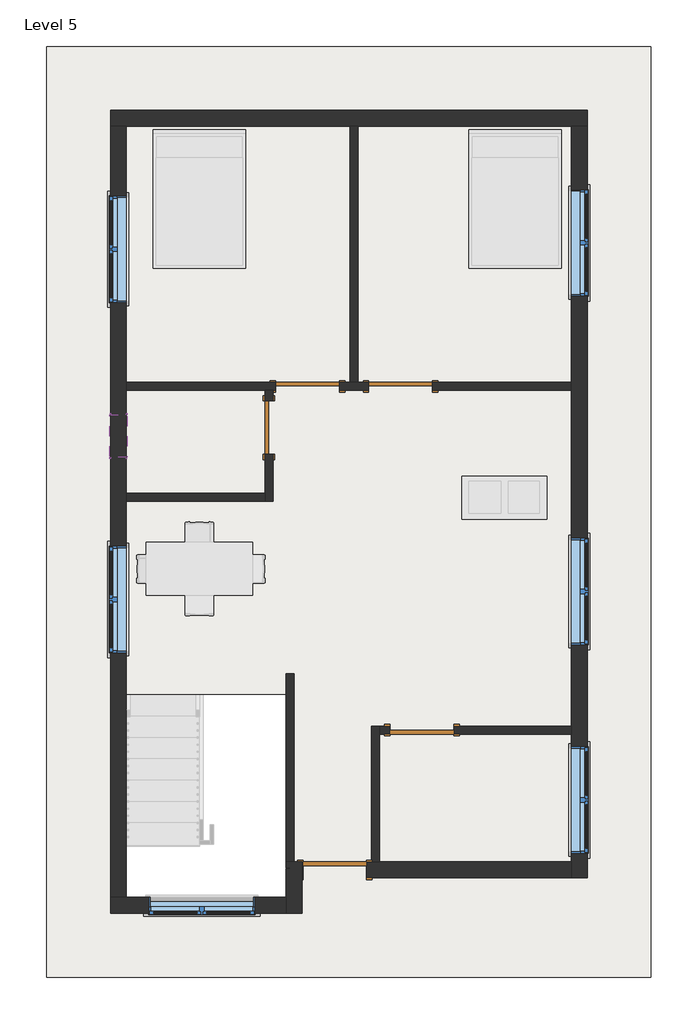
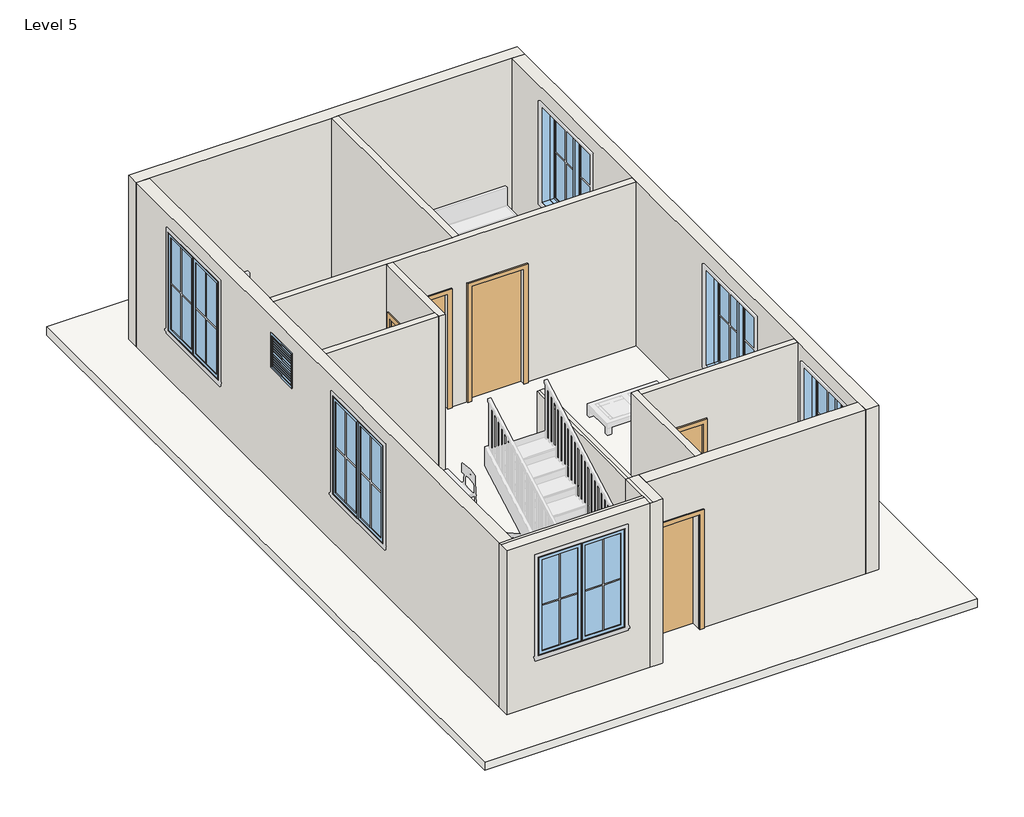
# One storey, part 1 of 3: 13 walls, 7 windows, 5 doors, 1 roof.
"""IFC4 building model written with IfcOpenShell, lengths in millimetres."""

from ifc_helpers import new_model, si_unit, frame, origin, place, context, project, spatial, polyline, outline, extrude, faceted_brep, transform, mapped, element, save
from components import door_214872d5, single_flush_door_3_e5f9f3c4, single_flush_door_3_305aa2a5, single_flush_door_3_0ca8825f, window_casement_double_win_5_f93960c7, window_f2d8fef0

model = new_model("IFC4")

# Units and contexts
model_context = context("Model", 3, world=origin())
ifc_project = project(units=[si_unit("LENGTHUNIT", "METRE", prefix="MILLI")], contexts=[model_context])

# Site, building, storey
site = spatial("IfcSite", under=ifc_project)
building = spatial("IfcBuilding", under=site)
storey = spatial("IfcBuildingStorey", under=building, Name="Level 5", Elevation=12649.2)

# Doors
placement = place(None, origin())
door_shape = door_214872d5(model_context)
element("IfcDoor", 1, ObjectType="Single-Flush : DOOR 2'6\"", at=placement, inside=storey, context=model_context, shape_type="MappedRepresentation", body=[
    mapped(door_shape, transform((-2193.930864, 251.0919982, 12649.2), x_axis=(0.0, 1.0, 0.0), y_axis=(-1.0, 0.0, 0.0), z_axis=(0.0, 0.0, 1.0))),
])
single_flush_door_3_shape = single_flush_door_3_e5f9f3c4(model_context)
element("IfcDoor", 2, ObjectType="Single-Flush : DOOR 3'", at=placement, inside=storey, context=model_context, shape_type="MappedRepresentation", body=[
    mapped(single_flush_door_3_shape, transform((-1641.3962678, 841.6419982, 12649.2), x_axis=(1.0, 0.0, 0.0), y_axis=(0.0, 1.0, 0.0), z_axis=(0.0, 0.0, 1.0))),
])
element("IfcDoor", 3, ObjectType="Single-Flush : DOOR 3'", at=placement, inside=storey, context=model_context, shape_type="MappedRepresentation", body=[
    mapped(single_flush_door_3_shape, transform((-3.180864, -4073.2580018, 12649.2), x_axis=(-1.0, 0.0, 0.0), y_axis=(0.0, -1.0, 0.0), z_axis=(0.0, 0.0, 1.0))),
])
single_flush_door_3_2_shape = single_flush_door_3_305aa2a5(model_context)
element("IfcDoor", 4, ObjectType="Single-Flush : DOOR 3'", at=placement, inside=storey, context=model_context, shape_type="MappedRepresentation", body=[
    mapped(single_flush_door_3_2_shape, transform((-307.980864, 841.6419982, 12649.2), x_axis=(-1.0, 0.0, 0.0), y_axis=(0.0, -1.0, 0.0), z_axis=(0.0, 0.0, 1.0))),
])
single_flush_door_3_3_shape = single_flush_door_3_0ca8825f(model_context)
element("IfcDoor", 5, ObjectType="Single-Flush : DOOR 3'", at=placement, inside=storey, context=model_context, shape_type="MappedRepresentation", body=[
    mapped(single_flush_door_3_3_shape, transform((-1250.955864, -6073.5080018, 12649.2), x_axis=(1.0, 0.0, 0.0), y_axis=(0.0, 1.0, 0.0), z_axis=(0.0, 0.0, 1.0))),
])

# Roof
element("IfcRoof", 6, ObjectType="ROOF 6\"", at=placement, inside=storey, context=model_context, shape_type="SweptSolid", body=[
    extrude(outline(polyline([(3273.419136, 5699.3919982), (3273.419136, -7610.2080018), (-5375.280864, -7610.2080018), (-5375.280864, 5699.3919982), (3273.419136, 5699.3919982)]), holes=[polyline([(-1895.480864, -3571.6080018), (-4232.280864, -3571.6080018), (-4232.280864, -6518.0080018), (-1895.480864, -6518.0080018), (-1895.480864, -3571.6080018)])]), frame((0.0, 0.0, 12496.8), z_axis=(0.0, 0.0, 1.0), x_axis=(1.0, 0.0, 0.0)), (0.0, 0.0, 1.0), 152.4),
])

# Walls
element("IfcWall", 7, ObjectType="WALL 4.5\"", at=placement, inside=storey, context=model_context, shape_type="SweptSolid", body=[
    extrude(outline(polyline([(-1031.880864, 898.7919982), (-1031.880864, 4556.3919982), (-917.580864, 4556.3919982), (-917.580864, 898.7919982), (-1031.880864, 898.7919982)])), frame((0.0, 0.0, 12649.2), z_axis=(0.0, 0.0, 1.0), x_axis=(1.0, 0.0, 0.0)), (0.0, 0.0, 1.0), 3048.0),
])
element("IfcWall", 8, ObjectType="WALL 4.5\"", at=placement, inside=storey, context=model_context, shape_type="Brep", body=[
    faceted_brep([(-765.180864, 898.7919982, 14782.8), (-765.180864, 898.7919982, 12649.2), (-917.580864, 898.7919982, 12649.2), (-1031.880864, 898.7919982, 12649.2), (-1184.1962678, 898.7919982, 12649.2), (-1184.1962678, 898.7919982, 14782.8), (-2098.5962678, 898.7919982, 14782.8), (-2098.5962678, 898.7919982, 12649.2), (-4232.280864, 898.7919982, 12649.2), (-4232.280864, 898.7919982, 15697.2), (-1031.880864, 898.7919982, 15697.2), (-917.580864, 898.7919982, 15697.2), (2130.419136, 898.7919982, 15697.2), (2130.419136, 898.7919982, 12649.2), (149.219136, 898.7919982, 12649.2), (149.219136, 898.7919982, 14782.8), (-1184.1962678, 784.4919982, 12649.2), (-765.180864, 784.4919982, 12649.2), (-765.180864, 784.4919982, 14782.8), (149.219136, 784.4919982, 14782.8), (149.219136, 784.4919982, 12649.2), (2130.419136, 784.4919982, 12649.2), (2130.419136, 784.4919982, 15697.2), (-2136.780864, 784.4919982, 15697.2), (-2251.080864, 784.4919982, 15697.2), (-4232.280864, 784.4919982, 15697.2), (-4232.280864, 784.4919982, 12649.2), (-2251.080864, 784.4919982, 12649.2), (-2136.780864, 784.4919982, 12649.2), (-2098.5962678, 784.4919982, 12649.2), (-2098.5962678, 784.4919982, 14782.8), (-1184.1962678, 784.4919982, 14782.8)], [[[0, 1, 2, 3, 4, 5, 6, 7, 8, 9, 10, 11, 12, 13, 14, 15]], [[16, 17, 18, 19, 20, 21, 22, 23, 24, 25, 26, 27, 28, 29, 30, 31]], [[29, 28, 27, 26, 8, 7]], [[14, 13, 21, 20]], [[4, 3, 2, 1, 17, 16]], [[13, 12, 22, 21]], [[9, 8, 26, 25]], [[5, 4, 16, 31]], [[6, 5, 31, 30]], [[7, 6, 30, 29]], [[18, 17, 1, 0]], [[19, 18, 0, 15]], [[20, 19, 15, 14]], [[12, 11, 10, 9, 25, 24, 23, 22]]]),
])
element("IfcWall", 9, ObjectType="WALL 4.5\"", at=placement, inside=storey, context=model_context, shape_type="Brep", body=[
    faceted_brep([(-2251.080864, 784.4919982, 12649.2), (-2251.080864, 632.0919982, 12649.2), (-2251.080864, 632.0919982, 14782.8), (-2251.080864, -129.9080018, 14782.8), (-2251.080864, -129.9080018, 12649.2), (-2251.080864, -688.7080018, 12649.2), (-2251.080864, -803.0080018, 12649.2), (-2251.080864, -803.0080018, 15697.2), (-2251.080864, -688.7080018, 15697.2), (-2251.080864, 784.4919982, 15697.2), (-2136.780864, 632.0919982, 14782.8), (-2136.780864, 632.0919982, 12649.2), (-2136.780864, 784.4919982, 12649.2), (-2136.780864, 784.4919982, 15697.2), (-2136.780864, -803.0080018, 15697.2), (-2136.780864, -803.0080018, 12649.2), (-2136.780864, -129.9080018, 12649.2), (-2136.780864, -129.9080018, 14782.8)], [[[0, 1, 2, 3, 4, 5, 6, 7, 8, 9]], [[10, 11, 12, 13, 14, 15, 16, 17]], [[16, 15, 6, 5, 4]], [[12, 11, 1, 0]], [[0, 9, 13, 12]], [[7, 6, 15, 14]], [[2, 1, 11, 10]], [[3, 2, 10, 17]], [[4, 3, 17, 16]], [[9, 8, 7, 14, 13]]]),
])
element("IfcWall", 10, ObjectType="WALL 4.5\"", at=placement, inside=storey, context=model_context, shape_type="SweptSolid", body=[
    extrude(outline(polyline([(-4232.280864, -688.7080018), (-2251.080864, -688.7080018), (-2251.080864, -803.0080018), (-4232.280864, -803.0080018), (-4232.280864, -688.7080018)])), frame((0.0, 0.0, 12649.2), z_axis=(0.0, 0.0, 1.0), x_axis=(1.0, 0.0, 0.0)), (0.0, 0.0, 1.0), 3048.0),
])
element("IfcWall", 11, ObjectType="WALL 4.5\"", at=placement, inside=storey, context=model_context, shape_type="Brep", body=[
    faceted_brep([(-1831.980864, -5959.2080018, 12649.2), (-1831.980864, -3266.8080018, 12649.2), (-1831.980864, -3266.8080018, 15697.2), (-1831.980864, -5959.2080018, 15697.2), (-1946.280864, -5959.2080018, 12649.2), (-1946.280864, -5959.2080018, 15697.2), (-1946.280864, -3266.8080018, 15697.2), (-1946.280864, -3266.8080018, 12649.2), (-1895.480864, -3266.8080018, 15697.2), (-1895.480864, -5959.2080018, 15697.2), (-1895.480864, -3571.6080018, 15697.2)], [[[0, 1, 2, 3]], [[4, 5, 6, 7]], [[1, 0, 4, 7]], [[2, 1, 7, 6, 8]], [[0, 3, 9, 5, 4]], [[3, 2, 8, 10, 9]], [[8, 6, 5, 9, 10]]]),
])
element("IfcWall", 12, ObjectType="WALL 4.5\"", at=placement, inside=storey, context=model_context, shape_type="Brep", body=[
    faceted_brep([(-612.780864, -5959.2080018, 12649.2), (-612.780864, -4130.4080018, 12649.2), (-612.780864, -4016.1080018, 12649.2), (-612.780864, -4016.1080018, 15697.2), (-612.780864, -4130.4080018, 15697.2), (-612.780864, -5959.2080018, 15697.2), (-727.080864, -5959.2080018, 12649.2), (-727.080864, -5959.2080018, 15697.2), (-727.080864, -4016.1080018, 15697.2), (-727.080864, -4016.1080018, 12649.2)], [[[0, 1, 2, 3, 4, 5]], [[6, 7, 8, 9]], [[2, 1, 0, 6, 9]], [[0, 5, 7, 6]], [[3, 2, 9, 8]], [[5, 4, 3, 8, 7]]]),
])
element("IfcWall", 13, ObjectType="WALL 4.5\"", at=placement, inside=storey, context=model_context, shape_type="SweptSolid", body=[
    extrude(outline(polyline([(12649.2, -612.780864), (12649.2, -460.380864), (14782.8, -460.380864), (14782.8, 454.019136), (12649.2, 454.019136), (12649.2, 2130.419136), (15697.2, 2130.419136), (15697.2, -612.780864), (12649.2, -612.780864)])), frame((0.0, -4130.4080018, 0.0), z_axis=(0.0, 1.0, 0.0), x_axis=(0.0, 0.0, 1.0)), (0.0, 0.0, 1.0), 114.3),
])
element("IfcWall", 14, ObjectType="WALL 9\"", at=placement, inside=storey, context=model_context, shape_type="Brep", body=[
    faceted_brep([(-4460.880864, 4556.3919982, 12649.2), (-4232.280864, 4556.3919982, 12649.2), (-1031.880864, 4556.3919982, 12649.2), (-917.580864, 4556.3919982, 12649.2), (2130.419136, 4556.3919982, 12649.2), (2359.019136, 4556.3919982, 12649.2), (2359.019136, 4556.3919982, 15697.2), (2130.419136, 4556.3919982, 15697.2), (-917.580864, 4556.3919982, 15697.2), (-1031.880864, 4556.3919982, 15697.2), (-4232.280864, 4556.3919982, 15697.2), (-4460.880864, 4556.3919982, 15697.2), (-4460.880864, 4784.9919982, 12649.2), (-4460.880864, 4784.9919982, 15697.2), (2359.019136, 4784.9919982, 15697.2), (2359.019136, 4784.9919982, 12649.2)], [[[0, 1, 2, 3, 4, 5, 6, 7, 8, 9, 10, 11]], [[12, 13, 14, 15]], [[5, 4, 3, 2, 1, 0, 12, 15]], [[6, 5, 15, 14]], [[0, 11, 13, 12]], [[11, 10, 9, 8, 7, 6, 14, 13]]]),
])
element("IfcWall", 15, ObjectType="WALL 9\"", at=placement, inside=storey, context=model_context, shape_type="Brep", body=[
    faceted_brep([(2130.419136, 4556.3919982, 12649.2), (2130.419136, 898.7919982, 12649.2), (2130.419136, 784.4919982, 12649.2), (2130.419136, -4016.1080018, 12649.2), (2130.419136, -4130.4080018, 12649.2), (2130.419136, -5959.2080018, 12649.2), (2130.419136, -6187.8080018, 12649.2), (2130.419136, -6187.8080018, 15697.2), (2130.419136, -5959.2080018, 15697.2), (2130.419136, -4130.4080018, 15697.2), (2130.419136, -4016.1080018, 15697.2), (2130.419136, 784.4919982, 15697.2), (2130.419136, 898.7919982, 15697.2), (2130.419136, 4556.3919982, 15697.2), (2130.419136, -5835.3830018, 15392.4), (2130.419136, -5835.3830018, 13563.6), (2130.419136, -4311.3830018, 13563.6), (2130.419136, -4311.3830018, 15392.4), (2130.419136, -2854.0580018, 15392.4), (2130.419136, -2854.0580018, 13563.6), (2130.419136, -1330.0580018, 13563.6), (2130.419136, -1330.0580018, 15392.4), (2130.419136, 2130.6919982, 15392.4), (2130.419136, 2130.6919982, 13563.6), (2130.419136, 3654.6919982, 13563.6), (2130.419136, 3654.6919982, 15392.4), (2359.019136, 4556.3919982, 12649.2), (2359.019136, 4556.3919982, 15697.2), (2359.019136, -6187.8080018, 15697.2), (2359.019136, -6187.8080018, 12649.2), (2359.019136, -5835.3830018, 15392.4), (2359.019136, -4311.3830018, 15392.4), (2359.019136, -4311.3830018, 13563.6), (2359.019136, -5835.3830018, 13563.6), (2359.019136, -2854.0580018, 15392.4), (2359.019136, -1330.0580018, 15392.4), (2359.019136, -1330.0580018, 13563.6), (2359.019136, -2854.0580018, 13563.6), (2359.019136, 2130.6919982, 15392.4), (2359.019136, 3654.6919982, 15392.4), (2359.019136, 3654.6919982, 13563.6), (2359.019136, 2130.6919982, 13563.6)], [[[0, 1, 2, 3, 4, 5, 6, 7, 8, 9, 10, 11, 12, 13], [14, 15, 16, 17], [18, 19, 20, 21], [22, 23, 24, 25]], [[26, 27, 28, 29], [30, 31, 32, 33], [34, 35, 36, 37], [38, 39, 40, 41]], [[6, 5, 4, 3, 2, 1, 0, 26, 29]], [[0, 13, 27, 26]], [[7, 6, 29, 28]], [[15, 14, 30, 33]], [[16, 15, 33, 32]], [[17, 16, 32, 31]], [[14, 17, 31, 30]], [[19, 18, 34, 37]], [[20, 19, 37, 36]], [[21, 20, 36, 35]], [[18, 21, 35, 34]], [[23, 22, 38, 41]], [[24, 23, 41, 40]], [[25, 24, 40, 39]], [[22, 25, 39, 38]], [[13, 12, 11, 10, 9, 8, 7, 28, 27]]]),
])
element("IfcWall", 16, ObjectType="WALL 9\"", at=placement, inside=storey, context=model_context, shape_type="Brep", body=[
    faceted_brep([(2130.419136, -5959.2080018, 12649.2), (-612.780864, -5959.2080018, 12649.2), (-727.080864, -5959.2080018, 12649.2), (-793.755864, -5959.2080018, 12649.2), (-793.755864, -5959.2080018, 14782.8), (-1708.155864, -5959.2080018, 14782.8), (-1708.155864, -5959.2080018, 12649.2), (-1717.680864, -5959.2080018, 12649.2), (-1717.680864, -5959.2080018, 15697.2), (-727.080864, -5959.2080018, 15697.2), (-612.780864, -5959.2080018, 15697.2), (2130.419136, -5959.2080018, 15697.2), (-793.755864, -6187.8080018, 14782.8), (-793.755864, -6187.8080018, 12649.2), (2130.419136, -6187.8080018, 12649.2), (2130.419136, -6187.8080018, 15697.2), (-1717.680864, -6187.8080018, 15697.2), (-1717.680864, -6187.8080018, 12649.2), (-1708.155864, -6187.8080018, 12649.2), (-1708.155864, -6187.8080018, 14782.8)], [[[0, 1, 2, 3, 4, 5, 6, 7, 8, 9, 10, 11]], [[12, 13, 14, 15, 16, 17, 18, 19]], [[18, 17, 7, 6]], [[14, 13, 3, 2, 1, 0]], [[0, 11, 15, 14]], [[8, 7, 17, 16]], [[4, 3, 13, 12]], [[5, 4, 12, 19]], [[6, 5, 19, 18]], [[11, 10, 9, 8, 16, 15]]]),
])
element("IfcWall", 17, ObjectType="WALL 9\"", at=placement, inside=storey, context=model_context, shape_type="Brep", body=[
    faceted_brep([(-1946.280864, -5959.2080018, 12649.2), (-1946.280864, -6467.2080018, 12649.2), (-1946.280864, -6695.8080018, 12649.2), (-1946.280864, -6695.8080018, 15697.2), (-1946.280864, -6467.2080018, 15697.2), (-1946.280864, -5959.2080018, 15697.2), (-1717.680864, -5959.2080018, 12649.2), (-1717.680864, -5959.2080018, 15697.2), (-1717.680864, -6187.8080018, 15697.2), (-1717.680864, -6695.8080018, 15697.2), (-1717.680864, -6695.8080018, 12649.2), (-1717.680864, -6187.8080018, 12649.2), (-1831.980864, -5959.2080018, 12649.2), (-1895.480864, -5959.2080018, 15697.2), (-1831.980864, -5959.2080018, 15697.2), (-1895.480864, -6695.8080018, 15697.2), (-1895.480864, -6518.0080018, 15697.2)], [[[0, 1, 2, 3, 4, 5]], [[6, 7, 8, 9, 10, 11]], [[2, 1, 0, 12, 6, 11, 10]], [[0, 5, 13, 14, 7, 6, 12]], [[3, 2, 10, 9, 15]], [[5, 4, 3, 15, 16, 13]], [[15, 9, 8, 7, 14, 13, 16]]]),
])
element("IfcWall", 18, ObjectType="WALL 9\"", at=placement, inside=storey, context=model_context, shape_type="Brep", body=[
    faceted_brep([(-1946.280864, -6467.2080018, 12649.2), (-4232.280864, -6467.2080018, 12649.2), (-4460.880864, -6467.2080018, 12649.2), (-4460.880864, -6467.2080018, 15697.2), (-4232.280864, -6467.2080018, 15697.2), (-1946.280864, -6467.2080018, 15697.2), (-3914.780864, -6467.2080018, 15392.4), (-3914.780864, -6467.2080018, 13563.6), (-2390.780864, -6467.2080018, 13563.6), (-2390.780864, -6467.2080018, 15392.4), (-1946.280864, -6695.8080018, 12649.2), (-1946.280864, -6695.8080018, 15697.2), (-4460.880864, -6695.8080018, 15697.2), (-4460.880864, -6695.8080018, 12649.2), (-3914.780864, -6695.8080018, 15392.4), (-2390.780864, -6695.8080018, 15392.4), (-2390.780864, -6695.8080018, 13563.6), (-3914.780864, -6695.8080018, 13563.6), (-1946.280864, -6518.0080018, 15697.2), (-4460.880864, -6518.0080018, 15697.2), (-4232.280864, -6518.0080018, 15697.2)], [[[0, 1, 2, 3, 4, 5], [6, 7, 8, 9]], [[10, 11, 12, 13], [14, 15, 16, 17]], [[2, 1, 0, 10, 13]], [[0, 5, 18, 11, 10]], [[3, 2, 13, 12, 19]], [[7, 6, 14, 17]], [[8, 7, 17, 16]], [[9, 8, 16, 15]], [[6, 9, 15, 14]], [[5, 4, 3, 19, 20, 18]], [[19, 12, 11, 18, 20]]]),
])
element("IfcWall", 19, ObjectType="WALL 9\"", at=placement, inside=storey, context=model_context, shape_type="Brep", body=[
    faceted_brep([(-4232.280864, -6467.2080018, 12649.2), (-4232.280864, -803.0080018, 12649.2), (-4232.280864, -688.7080018, 12649.2), (-4232.280864, 784.4919982, 12649.2), (-4232.280864, 898.7919982, 12649.2), (-4232.280864, 4556.3919982, 12649.2), (-4232.280864, 4556.3919982, 15697.2), (-4232.280864, 898.7919982, 15697.2), (-4232.280864, 784.4919982, 15697.2), (-4232.280864, -688.7080018, 15697.2), (-4232.280864, -803.0080018, 15697.2), (-4232.280864, -3571.6080018, 15697.2), (-4232.280864, -6467.2080018, 15697.2), (-4232.280864, -1445.1400081, 15392.4), (-4232.280864, -1445.1400081, 13563.6), (-4232.280864, -2969.1400081, 13563.6), (-4232.280864, -2969.1400081, 15392.4), (-4232.280864, 3562.6287133, 15392.4), (-4232.280864, 3562.6287133, 13563.6), (-4232.280864, 2038.6287133, 13563.6), (-4232.280864, 2038.6287133, 15392.4), (-4232.280864, -174.3580018, 15392.4), (-4232.280864, 435.2419982, 15392.4), (-4232.280864, 435.2419982, 14782.8), (-4232.280864, -174.3580018, 14782.8), (-4460.880864, -6467.2080018, 12649.2), (-4460.880864, -6467.2080018, 15697.2), (-4460.880864, 4556.3919982, 15697.2), (-4460.880864, 4556.3919982, 12649.2), (-4460.880864, -1445.1400081, 15392.4), (-4460.880864, -2969.1400081, 15392.4), (-4460.880864, -2969.1400081, 13563.6), (-4460.880864, -1445.1400081, 13563.6), (-4460.880864, 3562.6287133, 15392.4), (-4460.880864, 2038.6287133, 15392.4), (-4460.880864, 2038.6287133, 13563.6), (-4460.880864, 3562.6287133, 13563.6), (-4460.880864, -174.3580018, 15392.4), (-4460.880864, -174.3580018, 14782.8), (-4460.880864, 435.2419982, 14782.8), (-4460.880864, 435.2419982, 15392.4)], [[[0, 1, 2, 3, 4, 5, 6, 7, 8, 9, 10, 11, 12], [13, 14, 15, 16], [17, 18, 19, 20], [21, 22, 23, 24]], [[25, 26, 27, 28], [29, 30, 31, 32], [33, 34, 35, 36], [37, 38, 39, 40]], [[5, 4, 3, 2, 1, 0, 25, 28]], [[6, 5, 28, 27]], [[0, 12, 26, 25]], [[14, 13, 29, 32]], [[15, 14, 32, 31]], [[16, 15, 31, 30]], [[13, 16, 30, 29]], [[18, 17, 33, 36]], [[19, 18, 36, 35]], [[20, 19, 35, 34]], [[17, 20, 34, 33]], [[38, 37, 21, 24]], [[39, 38, 24, 23]], [[40, 39, 23, 22]], [[37, 40, 22, 21]], [[12, 11, 10, 9, 8, 7, 6, 27, 26]]]),
])

# Windows
window_casement_double_win_5_shape = window_casement_double_win_5_f93960c7(model_context)
element("IfcWindow", 20, ObjectType="Window-Casement-Double : WIN 5'", at=placement, inside=storey, context=model_context, shape_type="MappedRepresentation", body=[
    mapped(window_casement_double_win_5_shape, transform((-3152.780864, -6581.5080018, 12649.2), x_axis=(-1.0, 0.0, 0.0), y_axis=(0.0, -1.0, 0.0), z_axis=(0.0, 0.0, 1.0))),
])
element("IfcWindow", 21, ObjectType="Window-Casement-Double : WIN 5'", at=placement, inside=storey, context=model_context, shape_type="MappedRepresentation", body=[
    mapped(window_casement_double_win_5_shape, transform((2244.719136, -5073.3830018, 12649.2), x_axis=(0.0, -1.0, 0.0), y_axis=(1.0, 0.0, 0.0), z_axis=(0.0, 0.0, 1.0))),
])
element("IfcWindow", 22, ObjectType="Window-Casement-Double : WIN 5'", at=placement, inside=storey, context=model_context, shape_type="MappedRepresentation", body=[
    mapped(window_casement_double_win_5_shape, transform((2244.719136, -2092.0580018, 12649.2), x_axis=(0.0, -1.0, 0.0), y_axis=(1.0, 0.0, 0.0), z_axis=(0.0, 0.0, 1.0))),
])
element("IfcWindow", 23, ObjectType="Window-Casement-Double : WIN 5'", at=placement, inside=storey, context=model_context, shape_type="MappedRepresentation", body=[
    mapped(window_casement_double_win_5_shape, transform((-4346.580864, -2207.1400081, 12649.2), x_axis=(0.0, 1.0, 0.0), y_axis=(-1.0, 0.0, 0.0), z_axis=(0.0, 0.0, 1.0))),
])
element("IfcWindow", 24, ObjectType="Window-Casement-Double : WIN 5'", at=placement, inside=storey, context=model_context, shape_type="MappedRepresentation", body=[
    mapped(window_casement_double_win_5_shape, transform((2244.719136, 2892.6919982, 12649.2), x_axis=(0.0, -1.0, 0.0), y_axis=(1.0, 0.0, 0.0), z_axis=(0.0, 0.0, 1.0))),
])
element("IfcWindow", 25, ObjectType="Window-Casement-Double : WIN 5'", at=placement, inside=storey, context=model_context, shape_type="MappedRepresentation", body=[
    mapped(window_casement_double_win_5_shape, transform((-4346.580864, 2800.6287133, 12649.2), x_axis=(0.0, 1.0, 0.0), y_axis=(-1.0, 0.0, 0.0), z_axis=(0.0, 0.0, 1.0))),
])
window_shape = window_f2d8fef0(model_context)
element("IfcWindow", 26, ObjectType="Window-Louvers : 24\" x 24\"", at=placement, inside=storey, context=model_context, shape_type="MappedRepresentation", body=[
    mapped(window_shape, transform((-4352.930864, 130.4419982, 13868.4), x_axis=(0.0, 1.0, 0.0), y_axis=(-1.0, 0.0, 0.0), z_axis=(0.0, 0.0, 1.0))),
])

save(model, "model.ifc")

# Revit data of these elements
# Type "Single-Flush : DOOR 2'6\""
#   Type Mark = "9"
#   Construction Type Id = "MDOOR"
#   Assembly Code = "C1020"
#   Analytic Construction = "Metal"
#   Thickness = 0' - 2"
#   Heat Transfer Coefficient (U) = 0.651978 BTU/(h·ft²·°F)
#   Height = 7' - 0"
#   Trim Projection Ext = 0' - 1"
#   Trim Projection Int = 0' - 1"
#   Trim Width = 0' - 3"
#   Width = 2' - 6"
#   Define Thermal Properties by = 1
#   Door Material = Door - Panel
#   Frame Material = Door - Frame
#   Visual Light Transmittance = 0
#   Solar Heat Gain Coefficient = 0
#   Function = (empty or 0)
#   Wall Closure = (empty or 0)
# Type "Single-Flush : DOOR 3'"
#   Type Mark = "8"
#   Construction Type Id = "MDOOR"
#   Assembly Code = "C1020"
#   Analytic Construction = "Metal"
#   Thickness = 0' - 2"
#   Heat Transfer Coefficient (U) = 0.651978 BTU/(h·ft²·°F)
#   Height = 7' - 0"
#   Trim Projection Ext = 0' - 1"
#   Trim Projection Int = 0' - 1"
#   Trim Width = 0' - 3"
#   Width = 3' - 0"
#   Define Thermal Properties by = 1
#   Door Material = Door - Panel
#   Frame Material = Door - Frame
#   Visual Light Transmittance = 0
#   Solar Heat Gain Coefficient = 0
#   Function = (empty or 0)
#   Wall Closure = (empty or 0)
# Type "ROOF 6\""
#   Assembly Code = "B1020"
#   Layers, outside or top first: 0' - 6" no material (function 1)
# Type "WALL 4.5\""
#   Assembly Code = "B2010"
#   Layers, outside or top first: 0' - 4 1/2" no material (function 1)
# Type "WALL 9\""
#   Assembly Code = "B2010"
#   Layers, outside or top first: 0' - 9" no material (function 1)
# Type "Window-Casement-Double : WIN 5'"
#   Type Mark = "18"
#   Fire Rating = "0.5h"
#   Assembly Code = "B2020100"
#   Analytic Construction = "Double glazing - domestic"
#   Frame Extension [instance default] = 0' - 0 1/4"
#   Window Inset [instance default] = 0' - 0"
#   Wall Thickness [instance default] = 0' - 6"
#   Interior Wall Closure [instance default] = 0' - 2 1/4"
#   Half Width = 2' - 6"
#   Visual Light Transmittance = 0.81
#   Thermal Resistance (R) = 1.8146 (h·ft²·°F)/BTU
#   Solar Heat Gain Coefficient = 0.76
#   Rough Width = 5' - 0 1/2"
#   Rough Height = 6' - 0 1/2"
#   Height = 6' - 0"
#   Heat Transfer Coefficient (U) = 0.5511 BTU/(h·ft²·°F)
#   Exterior Wall Closure [instance default] = 0' - 1 1/4"
#   Extension Jamb [instance default] = 0' - 2 1/4"
#   Default Sill Height = 3' - 0"
#   Width = 5' - 0"
#   Muntin Visibility = yes
#   Interior Trim Visibility [instance default] = yes
#   Exterior Trim Visibility [instance default] = yes
#   Extension Jamb Visibility [instance default] = yes
#   Interior Trim Material = Wood - Stained
#   Muntin Pattern = Muntin Pattern_2x2 : Muntin Pattern_2x2
#   Interior Trim = Trim-Window-Interior-Flat : Picture Frame
#   Interior Frame Material = Wood - Stained
#   Glass Panel Material = Glass
#   Exterior Trim Material = Clad - White
#   Exterior Trim = Trim-Window-Exterior-Flat : with Sill
#   Exterior Frame Material = Clad - White
#   Wall Closure = (empty or 0)
# Type "Window-Louvers : 24\" x 24\""
#   Type Mark = "19"
#   Construction Type Id = "GSP4R"
#   Assembly Code = "B20"
#   Analytic Construction = "1/8 in Pilkington single glazing"
#   Visual Light Transmittance = 0.9
#   Thermal Resistance (R) = 1.53941 (h·ft²·°F)/BTU
#   Solar Heat Gain Coefficient = 0.78
#   Max Height = 1' - 11.74264"
#   Height = 2' - 0"
#   Heat Transfer Coefficient (U) = 0.6496 BTU/(h·ft²·°F)
#   Blade Width [instance default] = 1' - 10 1/2"
#   Blade Vertical Thickness = 0' - 0.35355"
#   Blade Thickness = 0' - 0 1/4"
#   Blade Spacing = 0' - 1 1/2"
#   Blade Height = 0' - 1.85355"
#   Blade Depth = 0' - 3"
#   Blade Angle = 45.00°
#   Default Sill Height = 3' - 0"
#   Trim Projection_Exterior = 0' - 0 1/2"
#   Trim Projection_Interior = 0' - 0 1/2"
#   Trim Width_Exterior = 0' - 1 1/2"
#   Trim Width_Interior = 0' - 1 1/2"
#   Width = 2' - 0"
#   Max Blade Count = 12
#   Define Thermal Properties by = 1
#   Blade Count = 12
#   Frame Material = Birch
#   Louver Material = Birch
#   Trim Exterior Material = Birch
#   Trim Interior Material = Birch
#   Wall Closure = (empty or 0)
# Element 1 (IfcDoor, "Single-Flush : DOOR 2'6\"")
#   Phase Created = New Construction
#   Materials on its faces: "Door - Frame", "Door - Panel"
# Elements 2, 3, 4, 5 (IfcDoor, "Single-Flush : DOOR 3'")
#   Phase Created = New Construction
#   Materials on its faces: "Door - Frame", "Door - Panel"
# Element 6 (IfcRoof, "ROOF 6\"")
#   built-in parameter 1001705 = 41.5 (stored number, unit not read)
#   built-in parameter 1001701 = -0.5 (stored number, unit not read)
#   built-in parameter 1001710 = 33615
#   Phase Created = New Construction
#   Materials on its faces: "Copper", "Wood - Stained"
# Elements 7, 8, 9, 10, 12, 13 (IfcWall, "WALL 4.5\"")
#   Top Offset = 0' - 0"
#   Base Offset = 0' - 0"
#   Unconnected Height = 10' - 0"
#   wall height = 10' - 0"
#   Phase Created = New Construction
#   Base Constraint = Level 5
#   Materials on its faces: "Default Wall"
# Element 11 (IfcWall, "WALL 4.5\"")
#   Top Offset = 0' - 0"
#   Base Offset = 0' - 0"
#   Unconnected Height = 10' - 0"
#   wall height = 10' - 0"
#   Phase Created = New Construction
#   Base Constraint = Level 5
#   Materials on its faces: "Default Wall", "Copper"
# Elements 14, 15, 16 (IfcWall, "WALL 9\"")
#   Top Offset = 0' - 0"
#   Base Offset = 0' - 0"
#   Unconnected Height = 10' - 0"
#   wall height = 10' - 0"
#   Phase Created = New Construction
#   Base Constraint = Level 5
#   Materials on its faces: "Default Wall"
# Elements 17, 18, 19 (IfcWall, "WALL 9\"")
#   Top Offset = 0' - 0"
#   Base Offset = 0' - 0"
#   Unconnected Height = 10' - 0"
#   wall height = 10' - 0"
#   Phase Created = New Construction
#   Base Constraint = Level 5
#   Materials on its faces: "Default Wall", "Copper"
# Element 20 (IfcWindow, "Window-Casement-Double : WIN 5'")
#   Mark = "29"
#   Window Inset = 0' - 0"
#   Interior Wall Closure = 0' - 2 1/4"
#   Frame Extension = 0' - 0 1/4"
#   Exterior Wall Closure = 0' - 1 1/4"
#   Interior Trim Visibility = yes
#   Exterior Trim Visibility = yes
#   Phase Created = New Construction
#   Materials on its faces: "Wood - Stained", "Glass", "Clad - White"
# Element 21 (IfcWindow, "Window-Casement-Double : WIN 5'")
#   Mark = "30"
#   Window Inset = 0' - 0"
#   Interior Wall Closure = 0' - 2 1/4"
#   Frame Extension = 0' - 0 1/4"
#   Exterior Wall Closure = 0' - 1 1/4"
#   Interior Trim Visibility = yes
#   Exterior Trim Visibility = yes
#   Phase Created = New Construction
#   Materials on its faces: "Wood - Stained", "Glass", "Clad - White"
# Element 22 (IfcWindow, "Window-Casement-Double : WIN 5'")
#   Mark = "31"
#   Window Inset = 0' - 0"
#   Interior Wall Closure = 0' - 2 1/4"
#   Frame Extension = 0' - 0 1/4"
#   Exterior Wall Closure = 0' - 1 1/4"
#   Interior Trim Visibility = yes
#   Exterior Trim Visibility = yes
#   Phase Created = New Construction
#   Materials on its faces: "Wood - Stained", "Glass", "Clad - White"
# Element 23 (IfcWindow, "Window-Casement-Double : WIN 5'")
#   Mark = "32"
#   Window Inset = 0' - 0"
#   Interior Wall Closure = 0' - 2 1/4"
#   Frame Extension = 0' - 0 1/4"
#   Exterior Wall Closure = 0' - 1 1/4"
#   Interior Trim Visibility = yes
#   Exterior Trim Visibility = yes
#   Phase Created = New Construction
#   Materials on its faces: "Wood - Stained", "Glass", "Clad - White"
# Element 24 (IfcWindow, "Window-Casement-Double : WIN 5'")
#   Mark = "33"
#   Window Inset = 0' - 0"
#   Interior Wall Closure = 0' - 2 1/4"
#   Frame Extension = 0' - 0 1/4"
#   Exterior Wall Closure = 0' - 1 1/4"
#   Interior Trim Visibility = yes
#   Exterior Trim Visibility = yes
#   Phase Created = New Construction
#   Materials on its faces: "Wood - Stained", "Glass", "Clad - White"
# Element 25 (IfcWindow, "Window-Casement-Double : WIN 5'")
#   Mark = "34"
#   Window Inset = 0' - 0"
#   Interior Wall Closure = 0' - 2 1/4"
#   Frame Extension = 0' - 0 1/4"
#   Exterior Wall Closure = 0' - 1 1/4"
#   Interior Trim Visibility = yes
#   Exterior Trim Visibility = yes
#   Phase Created = New Construction
#   Materials on its faces: "Wood - Stained", "Glass", "Clad - White"
# Element 26 (IfcWindow, "Window-Louvers : 24\" x 24\"")
#   Mark = "35"
#   Blade Width = 1' - 10 1/2"
#   Phase Created = New Construction
#   Materials on its faces: "Birch"
# Materials
#   "Door - Panel": class "Wood", colour RGB 210 159 95, transparency 0, Cost = 0
#   "Door - Frame": colour RGB 118 70 51, transparency 0, Cost = 0
#   "Wood - Stained": class "Wood", colour RGB 224 178 126, transparency 0, Cost = 0
#   "Glass": class "Glass", colour RGB 0 128 192, transparency 0.75, Description = "Soda Lime Glass", Cost = 0
#   "Clad - White": class "Wood", colour RGB 242 242 238, transparency 0, Cost = 0
#   "Birch": class "Wood", colour RGB 224 178 126, transparency 0, Description = "Betula Alleghaniensis", Cost = 0
#   "Copper": class "Metal", colour RGB 0 0 0, transparency 0, Description = "Copper, matte finish", Cost = 0
#   "Default Wall": colour RGB 128 128 128, transparency 0, Cost = 0
